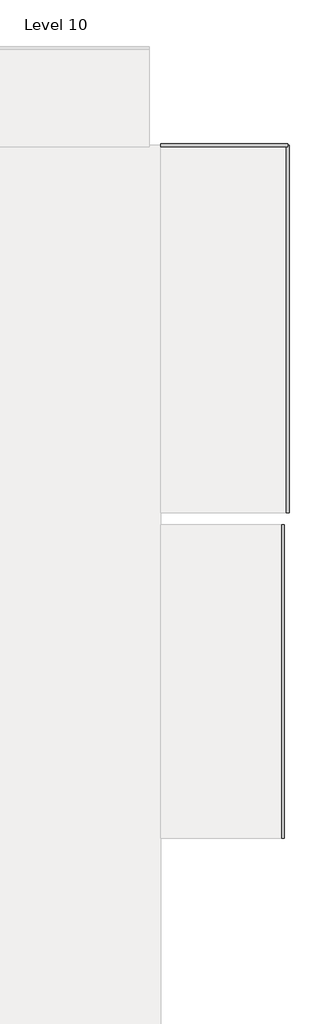
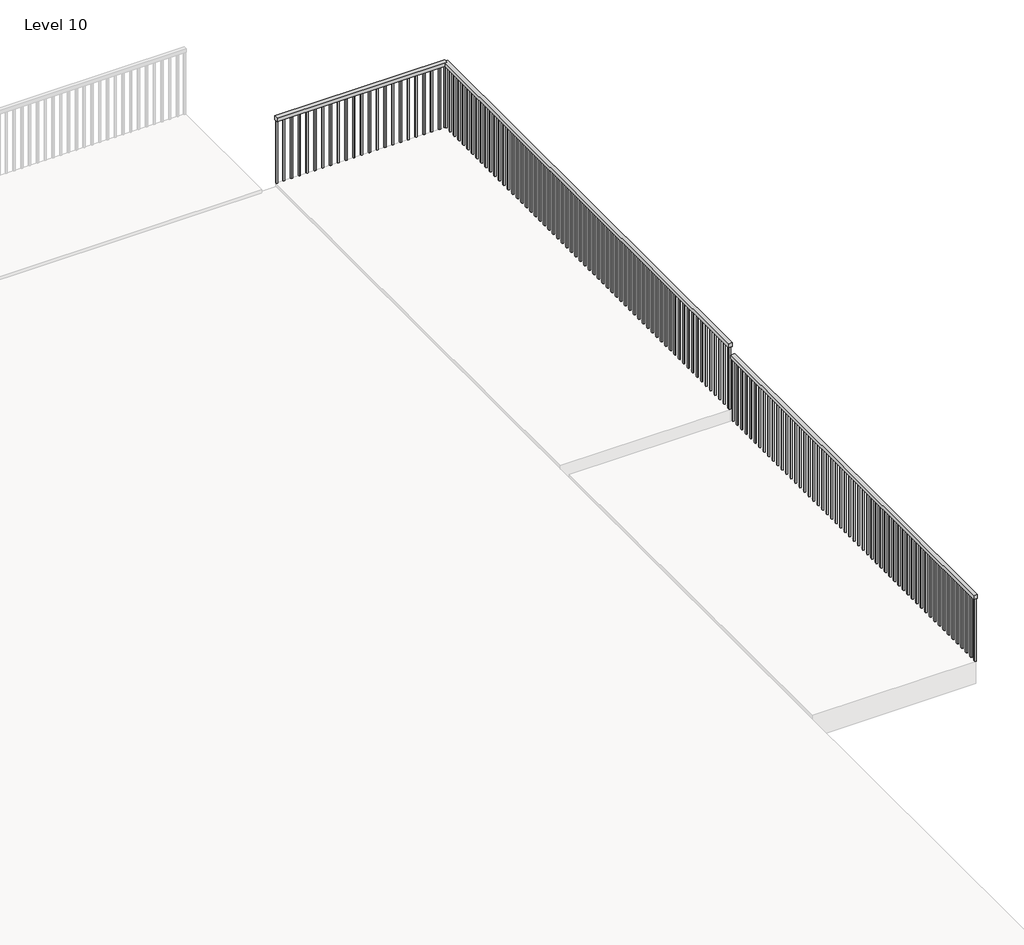
# One storey, part 4 of 5: 3 railings.
"""IFC4 building model written with IfcOpenShell, lengths in millimetres."""

from ifc_helpers import new_model, si_unit, frame, origin, place, context, project, spatial, polyline, outline, extrude, element, save

model = new_model("IFC4")

# Units and contexts
model_context = context("Model", 3, world=origin())
ifc_project = project(units=[si_unit("LENGTHUNIT", "METRE", prefix="MILLI")], contexts=[model_context])

# Site, building, storey
site = spatial("IfcSite", under=ifc_project)
building = spatial("IfcBuilding", under=site)
storey = spatial("IfcBuildingStorey", under=building, Name="Level 10", Elevation=12496.8)

# Railings
placement = place(None, origin())
element("IfcRailing", 1, ObjectType="Handrail - Rectangular", at=placement, inside=storey, context=model_context, shape_type="SweptSolid", body=[
    extrude(outline(polyline([(14106.5361222, 14772.744107), (14106.5361222, 14823.544107), (16321.4289933, 14823.544107), (16321.4289933, 14772.744107), (14106.5361222, 14772.744107)])), frame((0.0, 0.0, 13360.4), z_axis=(0.0, 0.0, 1.0), x_axis=(1.0, 0.0, 0.0)), (0.0, 0.0, 1.0), 50.8),
    extrude(outline(polyline([(16230.6111222, 14788.619107), (16230.6111222, 14807.669107), (16249.6611222, 14807.669107), (16249.6611222, 14788.619107), (16230.6111222, 14788.619107)])), frame((0.0, 0.0, 12496.8), z_axis=(0.0, 0.0, 1.0), x_axis=(1.0, 0.0, 0.0)), (0.0, 0.0, 1.0), 863.6),
    extrude(outline(polyline([(16129.0111222, 14788.619107), (16129.0111222, 14807.669107), (16148.0611222, 14807.669107), (16148.0611222, 14788.619107), (16129.0111222, 14788.619107)])), frame((0.0, 0.0, 12496.8), z_axis=(0.0, 0.0, 1.0), x_axis=(1.0, 0.0, 0.0)), (0.0, 0.0, 1.0), 863.6),
    extrude(outline(polyline([(16027.4111222, 14788.619107), (16027.4111222, 14807.669107), (16046.4611222, 14807.669107), (16046.4611222, 14788.619107), (16027.4111222, 14788.619107)])), frame((0.0, 0.0, 12496.8), z_axis=(0.0, 0.0, 1.0), x_axis=(1.0, 0.0, 0.0)), (0.0, 0.0, 1.0), 863.6),
    extrude(outline(polyline([(15925.8111222, 14788.619107), (15925.8111222, 14807.669107), (15944.8611222, 14807.669107), (15944.8611222, 14788.619107), (15925.8111222, 14788.619107)])), frame((0.0, 0.0, 12496.8), z_axis=(0.0, 0.0, 1.0), x_axis=(1.0, 0.0, 0.0)), (0.0, 0.0, 1.0), 863.6),
    extrude(outline(polyline([(15824.2111222, 14788.619107), (15824.2111222, 14807.669107), (15843.2611222, 14807.669107), (15843.2611222, 14788.619107), (15824.2111222, 14788.619107)])), frame((0.0, 0.0, 12496.8), z_axis=(0.0, 0.0, 1.0), x_axis=(1.0, 0.0, 0.0)), (0.0, 0.0, 1.0), 863.6),
    extrude(outline(polyline([(15722.6111222, 14788.619107), (15722.6111222, 14807.669107), (15741.6611222, 14807.669107), (15741.6611222, 14788.619107), (15722.6111222, 14788.619107)])), frame((0.0, 0.0, 12496.8), z_axis=(0.0, 0.0, 1.0), x_axis=(1.0, 0.0, 0.0)), (0.0, 0.0, 1.0), 863.6),
    extrude(outline(polyline([(15621.0111222, 14788.619107), (15621.0111222, 14807.669107), (15640.0611222, 14807.669107), (15640.0611222, 14788.619107), (15621.0111222, 14788.619107)])), frame((0.0, 0.0, 12496.8), z_axis=(0.0, 0.0, 1.0), x_axis=(1.0, 0.0, 0.0)), (0.0, 0.0, 1.0), 863.6),
    extrude(outline(polyline([(15519.4111222, 14788.619107), (15519.4111222, 14807.669107), (15538.4611222, 14807.669107), (15538.4611222, 14788.619107), (15519.4111222, 14788.619107)])), frame((0.0, 0.0, 12496.8), z_axis=(0.0, 0.0, 1.0), x_axis=(1.0, 0.0, 0.0)), (0.0, 0.0, 1.0), 863.6),
    extrude(outline(polyline([(15417.8111222, 14788.619107), (15417.8111222, 14807.669107), (15436.8611222, 14807.669107), (15436.8611222, 14788.619107), (15417.8111222, 14788.619107)])), frame((0.0, 0.0, 12496.8), z_axis=(0.0, 0.0, 1.0), x_axis=(1.0, 0.0, 0.0)), (0.0, 0.0, 1.0), 863.6),
    extrude(outline(polyline([(15316.2111222, 14788.619107), (15316.2111222, 14807.669107), (15335.2611222, 14807.669107), (15335.2611222, 14788.619107), (15316.2111222, 14788.619107)])), frame((0.0, 0.0, 12496.8), z_axis=(0.0, 0.0, 1.0), x_axis=(1.0, 0.0, 0.0)), (0.0, 0.0, 1.0), 863.6),
    extrude(outline(polyline([(15214.6111222, 14788.619107), (15214.6111222, 14807.669107), (15233.6611222, 14807.669107), (15233.6611222, 14788.619107), (15214.6111222, 14788.619107)])), frame((0.0, 0.0, 12496.8), z_axis=(0.0, 0.0, 1.0), x_axis=(1.0, 0.0, 0.0)), (0.0, 0.0, 1.0), 863.6),
    extrude(outline(polyline([(15113.0111222, 14788.619107), (15113.0111222, 14807.669107), (15132.0611222, 14807.669107), (15132.0611222, 14788.619107), (15113.0111222, 14788.619107)])), frame((0.0, 0.0, 12496.8), z_axis=(0.0, 0.0, 1.0), x_axis=(1.0, 0.0, 0.0)), (0.0, 0.0, 1.0), 863.6),
    extrude(outline(polyline([(15011.4111222, 14788.619107), (15011.4111222, 14807.669107), (15030.4611222, 14807.669107), (15030.4611222, 14788.619107), (15011.4111222, 14788.619107)])), frame((0.0, 0.0, 12496.8), z_axis=(0.0, 0.0, 1.0), x_axis=(1.0, 0.0, 0.0)), (0.0, 0.0, 1.0), 863.6),
    extrude(outline(polyline([(14909.8111222, 14788.619107), (14909.8111222, 14807.669107), (14928.8611222, 14807.669107), (14928.8611222, 14788.619107), (14909.8111222, 14788.619107)])), frame((0.0, 0.0, 12496.8), z_axis=(0.0, 0.0, 1.0), x_axis=(1.0, 0.0, 0.0)), (0.0, 0.0, 1.0), 863.6),
    extrude(outline(polyline([(14808.2111222, 14788.619107), (14808.2111222, 14807.669107), (14827.2611222, 14807.669107), (14827.2611222, 14788.619107), (14808.2111222, 14788.619107)])), frame((0.0, 0.0, 12496.8), z_axis=(0.0, 0.0, 1.0), x_axis=(1.0, 0.0, 0.0)), (0.0, 0.0, 1.0), 863.6),
    extrude(outline(polyline([(14706.6111222, 14788.619107), (14706.6111222, 14807.669107), (14725.6611222, 14807.669107), (14725.6611222, 14788.619107), (14706.6111222, 14788.619107)])), frame((0.0, 0.0, 12496.8), z_axis=(0.0, 0.0, 1.0), x_axis=(1.0, 0.0, 0.0)), (0.0, 0.0, 1.0), 863.6),
    extrude(outline(polyline([(14605.0111222, 14788.619107), (14605.0111222, 14807.669107), (14624.0611222, 14807.669107), (14624.0611222, 14788.619107), (14605.0111222, 14788.619107)])), frame((0.0, 0.0, 12496.8), z_axis=(0.0, 0.0, 1.0), x_axis=(1.0, 0.0, 0.0)), (0.0, 0.0, 1.0), 863.6),
    extrude(outline(polyline([(14503.4111222, 14788.619107), (14503.4111222, 14807.669107), (14522.4611222, 14807.669107), (14522.4611222, 14788.619107), (14503.4111222, 14788.619107)])), frame((0.0, 0.0, 12496.8), z_axis=(0.0, 0.0, 1.0), x_axis=(1.0, 0.0, 0.0)), (0.0, 0.0, 1.0), 863.6),
    extrude(outline(polyline([(14401.8111222, 14788.619107), (14401.8111222, 14807.669107), (14420.8611222, 14807.669107), (14420.8611222, 14788.619107), (14401.8111222, 14788.619107)])), frame((0.0, 0.0, 12496.8), z_axis=(0.0, 0.0, 1.0), x_axis=(1.0, 0.0, 0.0)), (0.0, 0.0, 1.0), 863.6),
    extrude(outline(polyline([(14300.2111222, 14788.619107), (14300.2111222, 14807.669107), (14319.2611222, 14807.669107), (14319.2611222, 14788.619107), (14300.2111222, 14788.619107)])), frame((0.0, 0.0, 12496.8), z_axis=(0.0, 0.0, 1.0), x_axis=(1.0, 0.0, 0.0)), (0.0, 0.0, 1.0), 863.6),
    extrude(outline(polyline([(14198.6111222, 14788.619107), (14198.6111222, 14807.669107), (14217.6611222, 14807.669107), (14217.6611222, 14788.619107), (14198.6111222, 14788.619107)])), frame((0.0, 0.0, 12496.8), z_axis=(0.0, 0.0, 1.0), x_axis=(1.0, 0.0, 0.0)), (0.0, 0.0, 1.0), 863.6),
    extrude(outline(polyline([(16302.3789933, 14788.619107), (16302.3789933, 14807.669107), (16321.4289933, 14807.669107), (16321.4289933, 14788.619107), (16302.3789933, 14788.619107)])), frame((0.0, 0.0, 12496.8), z_axis=(0.0, 0.0, 1.0), x_axis=(1.0, 0.0, 0.0)), (0.0, 0.0, 1.0), 863.6),
    extrude(outline(polyline([(14106.5361222, 14788.619107), (14106.5361222, 14807.669107), (14125.5861222, 14807.669107), (14125.5861222, 14788.619107), (14106.5361222, 14788.619107)])), frame((0.0, 0.0, 12496.8), z_axis=(0.0, 0.0, 1.0), x_axis=(1.0, 0.0, 0.0)), (0.0, 0.0, 1.0), 863.6),
])
element("IfcRailing", 2, ObjectType="Handrail - Rectangular", at=placement, inside=storey, context=model_context, shape_type="SweptSolid", body=[
    extrude(outline(polyline([(16296.0289933, 14798.144107), (16346.8289933, 14798.144107), (16346.8289933, 8367.8237525), (16296.0289933, 8367.8237525), (16296.0289933, 14798.144107)])), frame((0.0, 0.0, 13360.4), z_axis=(0.0, 0.0, 1.0), x_axis=(1.0, 0.0, 0.0)), (0.0, 0.0, 1.0), 50.8),
    extrude(outline(polyline([(16311.9039933, 8406.869107), (16330.9539933, 8406.869107), (16330.9539933, 8387.819107), (16311.9039933, 8387.819107), (16311.9039933, 8406.869107)])), frame((0.0, 0.0, 12496.8), z_axis=(0.0, 0.0, 1.0), x_axis=(1.0, 0.0, 0.0)), (0.0, 0.0, 1.0), 863.6),
    extrude(outline(polyline([(16311.9039933, 8508.469107), (16330.9539933, 8508.469107), (16330.9539933, 8489.419107), (16311.9039933, 8489.419107), (16311.9039933, 8508.469107)])), frame((0.0, 0.0, 12496.8), z_axis=(0.0, 0.0, 1.0), x_axis=(1.0, 0.0, 0.0)), (0.0, 0.0, 1.0), 863.6),
    extrude(outline(polyline([(16311.9039933, 8610.069107), (16330.9539933, 8610.069107), (16330.9539933, 8591.019107), (16311.9039933, 8591.019107), (16311.9039933, 8610.069107)])), frame((0.0, 0.0, 12496.8), z_axis=(0.0, 0.0, 1.0), x_axis=(1.0, 0.0, 0.0)), (0.0, 0.0, 1.0), 863.6),
    extrude(outline(polyline([(16311.9039933, 8711.669107), (16330.9539933, 8711.669107), (16330.9539933, 8692.619107), (16311.9039933, 8692.619107), (16311.9039933, 8711.669107)])), frame((0.0, 0.0, 12496.8), z_axis=(0.0, 0.0, 1.0), x_axis=(1.0, 0.0, 0.0)), (0.0, 0.0, 1.0), 863.6),
    extrude(outline(polyline([(16311.9039933, 8813.269107), (16330.9539933, 8813.269107), (16330.9539933, 8794.219107), (16311.9039933, 8794.219107), (16311.9039933, 8813.269107)])), frame((0.0, 0.0, 12496.8), z_axis=(0.0, 0.0, 1.0), x_axis=(1.0, 0.0, 0.0)), (0.0, 0.0, 1.0), 863.6),
    extrude(outline(polyline([(16311.9039933, 8914.869107), (16330.9539933, 8914.869107), (16330.9539933, 8895.819107), (16311.9039933, 8895.819107), (16311.9039933, 8914.869107)])), frame((0.0, 0.0, 12496.8), z_axis=(0.0, 0.0, 1.0), x_axis=(1.0, 0.0, 0.0)), (0.0, 0.0, 1.0), 863.6),
    extrude(outline(polyline([(16311.9039933, 9016.469107), (16330.9539933, 9016.469107), (16330.9539933, 8997.419107), (16311.9039933, 8997.419107), (16311.9039933, 9016.469107)])), frame((0.0, 0.0, 12496.8), z_axis=(0.0, 0.0, 1.0), x_axis=(1.0, 0.0, 0.0)), (0.0, 0.0, 1.0), 863.6),
    extrude(outline(polyline([(16311.9039933, 9118.069107), (16330.9539933, 9118.069107), (16330.9539933, 9099.019107), (16311.9039933, 9099.019107), (16311.9039933, 9118.069107)])), frame((0.0, 0.0, 12496.8), z_axis=(0.0, 0.0, 1.0), x_axis=(1.0, 0.0, 0.0)), (0.0, 0.0, 1.0), 863.6),
    extrude(outline(polyline([(16311.9039933, 9219.669107), (16330.9539933, 9219.669107), (16330.9539933, 9200.619107), (16311.9039933, 9200.619107), (16311.9039933, 9219.669107)])), frame((0.0, 0.0, 12496.8), z_axis=(0.0, 0.0, 1.0), x_axis=(1.0, 0.0, 0.0)), (0.0, 0.0, 1.0), 863.6),
    extrude(outline(polyline([(16311.9039933, 9321.269107), (16330.9539933, 9321.269107), (16330.9539933, 9302.219107), (16311.9039933, 9302.219107), (16311.9039933, 9321.269107)])), frame((0.0, 0.0, 12496.8), z_axis=(0.0, 0.0, 1.0), x_axis=(1.0, 0.0, 0.0)), (0.0, 0.0, 1.0), 863.6),
    extrude(outline(polyline([(16311.9039933, 9422.869107), (16330.9539933, 9422.869107), (16330.9539933, 9403.819107), (16311.9039933, 9403.819107), (16311.9039933, 9422.869107)])), frame((0.0, 0.0, 12496.8), z_axis=(0.0, 0.0, 1.0), x_axis=(1.0, 0.0, 0.0)), (0.0, 0.0, 1.0), 863.6),
    extrude(outline(polyline([(16311.9039933, 9524.469107), (16330.9539933, 9524.469107), (16330.9539933, 9505.419107), (16311.9039933, 9505.419107), (16311.9039933, 9524.469107)])), frame((0.0, 0.0, 12496.8), z_axis=(0.0, 0.0, 1.0), x_axis=(1.0, 0.0, 0.0)), (0.0, 0.0, 1.0), 863.6),
    extrude(outline(polyline([(16311.9039933, 9626.069107), (16330.9539933, 9626.069107), (16330.9539933, 9607.019107), (16311.9039933, 9607.019107), (16311.9039933, 9626.069107)])), frame((0.0, 0.0, 12496.8), z_axis=(0.0, 0.0, 1.0), x_axis=(1.0, 0.0, 0.0)), (0.0, 0.0, 1.0), 863.6),
    extrude(outline(polyline([(16311.9039933, 9727.669107), (16330.9539933, 9727.669107), (16330.9539933, 9708.619107), (16311.9039933, 9708.619107), (16311.9039933, 9727.669107)])), frame((0.0, 0.0, 12496.8), z_axis=(0.0, 0.0, 1.0), x_axis=(1.0, 0.0, 0.0)), (0.0, 0.0, 1.0), 863.6),
    extrude(outline(polyline([(16311.9039933, 9829.269107), (16330.9539933, 9829.269107), (16330.9539933, 9810.219107), (16311.9039933, 9810.219107), (16311.9039933, 9829.269107)])), frame((0.0, 0.0, 12496.8), z_axis=(0.0, 0.0, 1.0), x_axis=(1.0, 0.0, 0.0)), (0.0, 0.0, 1.0), 863.6),
    extrude(outline(polyline([(16311.9039933, 9930.869107), (16330.9539933, 9930.869107), (16330.9539933, 9911.819107), (16311.9039933, 9911.819107), (16311.9039933, 9930.869107)])), frame((0.0, 0.0, 12496.8), z_axis=(0.0, 0.0, 1.0), x_axis=(1.0, 0.0, 0.0)), (0.0, 0.0, 1.0), 863.6),
    extrude(outline(polyline([(16311.9039933, 10032.469107), (16330.9539933, 10032.469107), (16330.9539933, 10013.419107), (16311.9039933, 10013.419107), (16311.9039933, 10032.469107)])), frame((0.0, 0.0, 12496.8), z_axis=(0.0, 0.0, 1.0), x_axis=(1.0, 0.0, 0.0)), (0.0, 0.0, 1.0), 863.6),
    extrude(outline(polyline([(16311.9039933, 10134.069107), (16330.9539933, 10134.069107), (16330.9539933, 10115.019107), (16311.9039933, 10115.019107), (16311.9039933, 10134.069107)])), frame((0.0, 0.0, 12496.8), z_axis=(0.0, 0.0, 1.0), x_axis=(1.0, 0.0, 0.0)), (0.0, 0.0, 1.0), 863.6),
    extrude(outline(polyline([(16311.9039933, 10235.669107), (16330.9539933, 10235.669107), (16330.9539933, 10216.619107), (16311.9039933, 10216.619107), (16311.9039933, 10235.669107)])), frame((0.0, 0.0, 12496.8), z_axis=(0.0, 0.0, 1.0), x_axis=(1.0, 0.0, 0.0)), (0.0, 0.0, 1.0), 863.6),
    extrude(outline(polyline([(16311.9039933, 10337.269107), (16330.9539933, 10337.269107), (16330.9539933, 10318.219107), (16311.9039933, 10318.219107), (16311.9039933, 10337.269107)])), frame((0.0, 0.0, 12496.8), z_axis=(0.0, 0.0, 1.0), x_axis=(1.0, 0.0, 0.0)), (0.0, 0.0, 1.0), 863.6),
    extrude(outline(polyline([(16311.9039933, 10438.869107), (16330.9539933, 10438.869107), (16330.9539933, 10419.819107), (16311.9039933, 10419.819107), (16311.9039933, 10438.869107)])), frame((0.0, 0.0, 12496.8), z_axis=(0.0, 0.0, 1.0), x_axis=(1.0, 0.0, 0.0)), (0.0, 0.0, 1.0), 863.6),
    extrude(outline(polyline([(16311.9039933, 10540.469107), (16330.9539933, 10540.469107), (16330.9539933, 10521.419107), (16311.9039933, 10521.419107), (16311.9039933, 10540.469107)])), frame((0.0, 0.0, 12496.8), z_axis=(0.0, 0.0, 1.0), x_axis=(1.0, 0.0, 0.0)), (0.0, 0.0, 1.0), 863.6),
    extrude(outline(polyline([(16311.9039933, 10642.069107), (16330.9539933, 10642.069107), (16330.9539933, 10623.019107), (16311.9039933, 10623.019107), (16311.9039933, 10642.069107)])), frame((0.0, 0.0, 12496.8), z_axis=(0.0, 0.0, 1.0), x_axis=(1.0, 0.0, 0.0)), (0.0, 0.0, 1.0), 863.6),
    extrude(outline(polyline([(16311.9039933, 10743.669107), (16330.9539933, 10743.669107), (16330.9539933, 10724.619107), (16311.9039933, 10724.619107), (16311.9039933, 10743.669107)])), frame((0.0, 0.0, 12496.8), z_axis=(0.0, 0.0, 1.0), x_axis=(1.0, 0.0, 0.0)), (0.0, 0.0, 1.0), 863.6),
    extrude(outline(polyline([(16311.9039933, 10845.269107), (16330.9539933, 10845.269107), (16330.9539933, 10826.219107), (16311.9039933, 10826.219107), (16311.9039933, 10845.269107)])), frame((0.0, 0.0, 12496.8), z_axis=(0.0, 0.0, 1.0), x_axis=(1.0, 0.0, 0.0)), (0.0, 0.0, 1.0), 863.6),
    extrude(outline(polyline([(16311.9039933, 10946.869107), (16330.9539933, 10946.869107), (16330.9539933, 10927.819107), (16311.9039933, 10927.819107), (16311.9039933, 10946.869107)])), frame((0.0, 0.0, 12496.8), z_axis=(0.0, 0.0, 1.0), x_axis=(1.0, 0.0, 0.0)), (0.0, 0.0, 1.0), 863.6),
    extrude(outline(polyline([(16311.9039933, 11048.469107), (16330.9539933, 11048.469107), (16330.9539933, 11029.419107), (16311.9039933, 11029.419107), (16311.9039933, 11048.469107)])), frame((0.0, 0.0, 12496.8), z_axis=(0.0, 0.0, 1.0), x_axis=(1.0, 0.0, 0.0)), (0.0, 0.0, 1.0), 863.6),
    extrude(outline(polyline([(16311.9039933, 11150.069107), (16330.9539933, 11150.069107), (16330.9539933, 11131.019107), (16311.9039933, 11131.019107), (16311.9039933, 11150.069107)])), frame((0.0, 0.0, 12496.8), z_axis=(0.0, 0.0, 1.0), x_axis=(1.0, 0.0, 0.0)), (0.0, 0.0, 1.0), 863.6),
    extrude(outline(polyline([(16311.9039933, 11251.669107), (16330.9539933, 11251.669107), (16330.9539933, 11232.619107), (16311.9039933, 11232.619107), (16311.9039933, 11251.669107)])), frame((0.0, 0.0, 12496.8), z_axis=(0.0, 0.0, 1.0), x_axis=(1.0, 0.0, 0.0)), (0.0, 0.0, 1.0), 863.6),
    extrude(outline(polyline([(16311.9039933, 11353.269107), (16330.9539933, 11353.269107), (16330.9539933, 11334.219107), (16311.9039933, 11334.219107), (16311.9039933, 11353.269107)])), frame((0.0, 0.0, 12496.8), z_axis=(0.0, 0.0, 1.0), x_axis=(1.0, 0.0, 0.0)), (0.0, 0.0, 1.0), 863.6),
    extrude(outline(polyline([(16311.9039933, 11454.869107), (16330.9539933, 11454.869107), (16330.9539933, 11435.819107), (16311.9039933, 11435.819107), (16311.9039933, 11454.869107)])), frame((0.0, 0.0, 12496.8), z_axis=(0.0, 0.0, 1.0), x_axis=(1.0, 0.0, 0.0)), (0.0, 0.0, 1.0), 863.6),
    extrude(outline(polyline([(16311.9039933, 11556.469107), (16330.9539933, 11556.469107), (16330.9539933, 11537.419107), (16311.9039933, 11537.419107), (16311.9039933, 11556.469107)])), frame((0.0, 0.0, 12496.8), z_axis=(0.0, 0.0, 1.0), x_axis=(1.0, 0.0, 0.0)), (0.0, 0.0, 1.0), 863.6),
    extrude(outline(polyline([(16311.9039933, 11658.069107), (16330.9539933, 11658.069107), (16330.9539933, 11639.019107), (16311.9039933, 11639.019107), (16311.9039933, 11658.069107)])), frame((0.0, 0.0, 12496.8), z_axis=(0.0, 0.0, 1.0), x_axis=(1.0, 0.0, 0.0)), (0.0, 0.0, 1.0), 863.6),
    extrude(outline(polyline([(16311.9039933, 11759.669107), (16330.9539933, 11759.669107), (16330.9539933, 11740.619107), (16311.9039933, 11740.619107), (16311.9039933, 11759.669107)])), frame((0.0, 0.0, 12496.8), z_axis=(0.0, 0.0, 1.0), x_axis=(1.0, 0.0, 0.0)), (0.0, 0.0, 1.0), 863.6),
    extrude(outline(polyline([(16311.9039933, 11861.269107), (16330.9539933, 11861.269107), (16330.9539933, 11842.219107), (16311.9039933, 11842.219107), (16311.9039933, 11861.269107)])), frame((0.0, 0.0, 12496.8), z_axis=(0.0, 0.0, 1.0), x_axis=(1.0, 0.0, 0.0)), (0.0, 0.0, 1.0), 863.6),
    extrude(outline(polyline([(16311.9039933, 11962.869107), (16330.9539933, 11962.869107), (16330.9539933, 11943.819107), (16311.9039933, 11943.819107), (16311.9039933, 11962.869107)])), frame((0.0, 0.0, 12496.8), z_axis=(0.0, 0.0, 1.0), x_axis=(1.0, 0.0, 0.0)), (0.0, 0.0, 1.0), 863.6),
    extrude(outline(polyline([(16311.9039933, 12064.469107), (16330.9539933, 12064.469107), (16330.9539933, 12045.419107), (16311.9039933, 12045.419107), (16311.9039933, 12064.469107)])), frame((0.0, 0.0, 12496.8), z_axis=(0.0, 0.0, 1.0), x_axis=(1.0, 0.0, 0.0)), (0.0, 0.0, 1.0), 863.6),
    extrude(outline(polyline([(16311.9039933, 12166.069107), (16330.9539933, 12166.069107), (16330.9539933, 12147.019107), (16311.9039933, 12147.019107), (16311.9039933, 12166.069107)])), frame((0.0, 0.0, 12496.8), z_axis=(0.0, 0.0, 1.0), x_axis=(1.0, 0.0, 0.0)), (0.0, 0.0, 1.0), 863.6),
    extrude(outline(polyline([(16311.9039933, 12267.669107), (16330.9539933, 12267.669107), (16330.9539933, 12248.619107), (16311.9039933, 12248.619107), (16311.9039933, 12267.669107)])), frame((0.0, 0.0, 12496.8), z_axis=(0.0, 0.0, 1.0), x_axis=(1.0, 0.0, 0.0)), (0.0, 0.0, 1.0), 863.6),
    extrude(outline(polyline([(16311.9039933, 12369.269107), (16330.9539933, 12369.269107), (16330.9539933, 12350.219107), (16311.9039933, 12350.219107), (16311.9039933, 12369.269107)])), frame((0.0, 0.0, 12496.8), z_axis=(0.0, 0.0, 1.0), x_axis=(1.0, 0.0, 0.0)), (0.0, 0.0, 1.0), 863.6),
    extrude(outline(polyline([(16311.9039933, 12470.869107), (16330.9539933, 12470.869107), (16330.9539933, 12451.819107), (16311.9039933, 12451.819107), (16311.9039933, 12470.869107)])), frame((0.0, 0.0, 12496.8), z_axis=(0.0, 0.0, 1.0), x_axis=(1.0, 0.0, 0.0)), (0.0, 0.0, 1.0), 863.6),
    extrude(outline(polyline([(16311.9039933, 12572.469107), (16330.9539933, 12572.469107), (16330.9539933, 12553.419107), (16311.9039933, 12553.419107), (16311.9039933, 12572.469107)])), frame((0.0, 0.0, 12496.8), z_axis=(0.0, 0.0, 1.0), x_axis=(1.0, 0.0, 0.0)), (0.0, 0.0, 1.0), 863.6),
    extrude(outline(polyline([(16311.9039933, 12674.069107), (16330.9539933, 12674.069107), (16330.9539933, 12655.019107), (16311.9039933, 12655.019107), (16311.9039933, 12674.069107)])), frame((0.0, 0.0, 12496.8), z_axis=(0.0, 0.0, 1.0), x_axis=(1.0, 0.0, 0.0)), (0.0, 0.0, 1.0), 863.6),
    extrude(outline(polyline([(16311.9039933, 12775.669107), (16330.9539933, 12775.669107), (16330.9539933, 12756.619107), (16311.9039933, 12756.619107), (16311.9039933, 12775.669107)])), frame((0.0, 0.0, 12496.8), z_axis=(0.0, 0.0, 1.0), x_axis=(1.0, 0.0, 0.0)), (0.0, 0.0, 1.0), 863.6),
    extrude(outline(polyline([(16311.9039933, 12877.269107), (16330.9539933, 12877.269107), (16330.9539933, 12858.219107), (16311.9039933, 12858.219107), (16311.9039933, 12877.269107)])), frame((0.0, 0.0, 12496.8), z_axis=(0.0, 0.0, 1.0), x_axis=(1.0, 0.0, 0.0)), (0.0, 0.0, 1.0), 863.6),
    extrude(outline(polyline([(16311.9039933, 12978.869107), (16330.9539933, 12978.869107), (16330.9539933, 12959.819107), (16311.9039933, 12959.819107), (16311.9039933, 12978.869107)])), frame((0.0, 0.0, 12496.8), z_axis=(0.0, 0.0, 1.0), x_axis=(1.0, 0.0, 0.0)), (0.0, 0.0, 1.0), 863.6),
    extrude(outline(polyline([(16311.9039933, 13080.469107), (16330.9539933, 13080.469107), (16330.9539933, 13061.419107), (16311.9039933, 13061.419107), (16311.9039933, 13080.469107)])), frame((0.0, 0.0, 12496.8), z_axis=(0.0, 0.0, 1.0), x_axis=(1.0, 0.0, 0.0)), (0.0, 0.0, 1.0), 863.6),
    extrude(outline(polyline([(16311.9039933, 13182.069107), (16330.9539933, 13182.069107), (16330.9539933, 13163.019107), (16311.9039933, 13163.019107), (16311.9039933, 13182.069107)])), frame((0.0, 0.0, 12496.8), z_axis=(0.0, 0.0, 1.0), x_axis=(1.0, 0.0, 0.0)), (0.0, 0.0, 1.0), 863.6),
    extrude(outline(polyline([(16311.9039933, 13283.669107), (16330.9539933, 13283.669107), (16330.9539933, 13264.619107), (16311.9039933, 13264.619107), (16311.9039933, 13283.669107)])), frame((0.0, 0.0, 12496.8), z_axis=(0.0, 0.0, 1.0), x_axis=(1.0, 0.0, 0.0)), (0.0, 0.0, 1.0), 863.6),
    extrude(outline(polyline([(16311.9039933, 13385.269107), (16330.9539933, 13385.269107), (16330.9539933, 13366.219107), (16311.9039933, 13366.219107), (16311.9039933, 13385.269107)])), frame((0.0, 0.0, 12496.8), z_axis=(0.0, 0.0, 1.0), x_axis=(1.0, 0.0, 0.0)), (0.0, 0.0, 1.0), 863.6),
    extrude(outline(polyline([(16311.9039933, 13486.869107), (16330.9539933, 13486.869107), (16330.9539933, 13467.819107), (16311.9039933, 13467.819107), (16311.9039933, 13486.869107)])), frame((0.0, 0.0, 12496.8), z_axis=(0.0, 0.0, 1.0), x_axis=(1.0, 0.0, 0.0)), (0.0, 0.0, 1.0), 863.6),
    extrude(outline(polyline([(16311.9039933, 13588.469107), (16330.9539933, 13588.469107), (16330.9539933, 13569.419107), (16311.9039933, 13569.419107), (16311.9039933, 13588.469107)])), frame((0.0, 0.0, 12496.8), z_axis=(0.0, 0.0, 1.0), x_axis=(1.0, 0.0, 0.0)), (0.0, 0.0, 1.0), 863.6),
    extrude(outline(polyline([(16311.9039933, 13690.069107), (16330.9539933, 13690.069107), (16330.9539933, 13671.019107), (16311.9039933, 13671.019107), (16311.9039933, 13690.069107)])), frame((0.0, 0.0, 12496.8), z_axis=(0.0, 0.0, 1.0), x_axis=(1.0, 0.0, 0.0)), (0.0, 0.0, 1.0), 863.6),
    extrude(outline(polyline([(16311.9039933, 13791.669107), (16330.9539933, 13791.669107), (16330.9539933, 13772.619107), (16311.9039933, 13772.619107), (16311.9039933, 13791.669107)])), frame((0.0, 0.0, 12496.8), z_axis=(0.0, 0.0, 1.0), x_axis=(1.0, 0.0, 0.0)), (0.0, 0.0, 1.0), 863.6),
    extrude(outline(polyline([(16311.9039933, 13893.269107), (16330.9539933, 13893.269107), (16330.9539933, 13874.219107), (16311.9039933, 13874.219107), (16311.9039933, 13893.269107)])), frame((0.0, 0.0, 12496.8), z_axis=(0.0, 0.0, 1.0), x_axis=(1.0, 0.0, 0.0)), (0.0, 0.0, 1.0), 863.6),
    extrude(outline(polyline([(16311.9039933, 13994.869107), (16330.9539933, 13994.869107), (16330.9539933, 13975.819107), (16311.9039933, 13975.819107), (16311.9039933, 13994.869107)])), frame((0.0, 0.0, 12496.8), z_axis=(0.0, 0.0, 1.0), x_axis=(1.0, 0.0, 0.0)), (0.0, 0.0, 1.0), 863.6),
    extrude(outline(polyline([(16311.9039933, 14096.469107), (16330.9539933, 14096.469107), (16330.9539933, 14077.419107), (16311.9039933, 14077.419107), (16311.9039933, 14096.469107)])), frame((0.0, 0.0, 12496.8), z_axis=(0.0, 0.0, 1.0), x_axis=(1.0, 0.0, 0.0)), (0.0, 0.0, 1.0), 863.6),
    extrude(outline(polyline([(16311.9039933, 14198.069107), (16330.9539933, 14198.069107), (16330.9539933, 14179.019107), (16311.9039933, 14179.019107), (16311.9039933, 14198.069107)])), frame((0.0, 0.0, 12496.8), z_axis=(0.0, 0.0, 1.0), x_axis=(1.0, 0.0, 0.0)), (0.0, 0.0, 1.0), 863.6),
    extrude(outline(polyline([(16311.9039933, 14299.669107), (16330.9539933, 14299.669107), (16330.9539933, 14280.619107), (16311.9039933, 14280.619107), (16311.9039933, 14299.669107)])), frame((0.0, 0.0, 12496.8), z_axis=(0.0, 0.0, 1.0), x_axis=(1.0, 0.0, 0.0)), (0.0, 0.0, 1.0), 863.6),
    extrude(outline(polyline([(16311.9039933, 14401.269107), (16330.9539933, 14401.269107), (16330.9539933, 14382.219107), (16311.9039933, 14382.219107), (16311.9039933, 14401.269107)])), frame((0.0, 0.0, 12496.8), z_axis=(0.0, 0.0, 1.0), x_axis=(1.0, 0.0, 0.0)), (0.0, 0.0, 1.0), 863.6),
    extrude(outline(polyline([(16311.9039933, 14502.869107), (16330.9539933, 14502.869107), (16330.9539933, 14483.819107), (16311.9039933, 14483.819107), (16311.9039933, 14502.869107)])), frame((0.0, 0.0, 12496.8), z_axis=(0.0, 0.0, 1.0), x_axis=(1.0, 0.0, 0.0)), (0.0, 0.0, 1.0), 863.6),
    extrude(outline(polyline([(16311.9039933, 14604.469107), (16330.9539933, 14604.469107), (16330.9539933, 14585.419107), (16311.9039933, 14585.419107), (16311.9039933, 14604.469107)])), frame((0.0, 0.0, 12496.8), z_axis=(0.0, 0.0, 1.0), x_axis=(1.0, 0.0, 0.0)), (0.0, 0.0, 1.0), 863.6),
    extrude(outline(polyline([(16311.9039933, 14706.069107), (16330.9539933, 14706.069107), (16330.9539933, 14687.019107), (16311.9039933, 14687.019107), (16311.9039933, 14706.069107)])), frame((0.0, 0.0, 12496.8), z_axis=(0.0, 0.0, 1.0), x_axis=(1.0, 0.0, 0.0)), (0.0, 0.0, 1.0), 863.6),
    extrude(outline(polyline([(16311.9039933, 8386.8737525), (16330.9539933, 8386.8737525), (16330.9539933, 8367.8237525), (16311.9039933, 8367.8237525), (16311.9039933, 8386.8737525)])), frame((0.0, 0.0, 12496.8), z_axis=(0.0, 0.0, 1.0), x_axis=(1.0, 0.0, 0.0)), (0.0, 0.0, 1.0), 863.6),
    extrude(outline(polyline([(16311.9039933, 14798.144107), (16330.9539933, 14798.144107), (16330.9539933, 14779.094107), (16311.9039933, 14779.094107), (16311.9039933, 14798.144107)])), frame((0.0, 0.0, 12496.8), z_axis=(0.0, 0.0, 1.0), x_axis=(1.0, 0.0, 0.0)), (0.0, 0.0, 1.0), 863.6),
])
element("IfcRailing", 3, ObjectType="Handrail - Rectangular", at=placement, inside=storey, context=model_context, shape_type="SweptSolid", body=[
    extrude(outline(polyline([(16214.7361222, 8164.6237525), (16265.5361222, 8164.6237525), (16265.5361222, 2678.2237525), (16214.7361222, 2678.2237525), (16214.7361222, 8164.6237525)])), frame((0.0, 0.0, 13360.4), z_axis=(0.0, 0.0, 1.0), x_axis=(1.0, 0.0, 0.0)), (0.0, 0.0, 1.0), 50.8),
    extrude(outline(polyline([(16230.6111222, 2789.3487525), (16249.6611222, 2789.3487525), (16249.6611222, 2770.2987525), (16230.6111222, 2770.2987525), (16230.6111222, 2789.3487525)])), frame((0.0, 0.0, 12496.8), z_axis=(0.0, 0.0, 1.0), x_axis=(1.0, 0.0, 0.0)), (0.0, 0.0, 1.0), 863.6),
    extrude(outline(polyline([(16230.6111222, 2890.9487525), (16249.6611222, 2890.9487525), (16249.6611222, 2871.8987525), (16230.6111222, 2871.8987525), (16230.6111222, 2890.9487525)])), frame((0.0, 0.0, 12496.8), z_axis=(0.0, 0.0, 1.0), x_axis=(1.0, 0.0, 0.0)), (0.0, 0.0, 1.0), 863.6),
    extrude(outline(polyline([(16230.6111222, 2992.5487525), (16249.6611222, 2992.5487525), (16249.6611222, 2973.4987525), (16230.6111222, 2973.4987525), (16230.6111222, 2992.5487525)])), frame((0.0, 0.0, 12496.8), z_axis=(0.0, 0.0, 1.0), x_axis=(1.0, 0.0, 0.0)), (0.0, 0.0, 1.0), 863.6),
    extrude(outline(polyline([(16230.6111222, 3094.1487525), (16249.6611222, 3094.1487525), (16249.6611222, 3075.0987525), (16230.6111222, 3075.0987525), (16230.6111222, 3094.1487525)])), frame((0.0, 0.0, 12496.8), z_axis=(0.0, 0.0, 1.0), x_axis=(1.0, 0.0, 0.0)), (0.0, 0.0, 1.0), 863.6),
    extrude(outline(polyline([(16230.6111222, 3195.7487525), (16249.6611222, 3195.7487525), (16249.6611222, 3176.6987525), (16230.6111222, 3176.6987525), (16230.6111222, 3195.7487525)])), frame((0.0, 0.0, 12496.8), z_axis=(0.0, 0.0, 1.0), x_axis=(1.0, 0.0, 0.0)), (0.0, 0.0, 1.0), 863.6),
    extrude(outline(polyline([(16230.6111222, 3297.3487525), (16249.6611222, 3297.3487525), (16249.6611222, 3278.2987525), (16230.6111222, 3278.2987525), (16230.6111222, 3297.3487525)])), frame((0.0, 0.0, 12496.8), z_axis=(0.0, 0.0, 1.0), x_axis=(1.0, 0.0, 0.0)), (0.0, 0.0, 1.0), 863.6),
    extrude(outline(polyline([(16230.6111222, 3398.9487525), (16249.6611222, 3398.9487525), (16249.6611222, 3379.8987525), (16230.6111222, 3379.8987525), (16230.6111222, 3398.9487525)])), frame((0.0, 0.0, 12496.8), z_axis=(0.0, 0.0, 1.0), x_axis=(1.0, 0.0, 0.0)), (0.0, 0.0, 1.0), 863.6),
    extrude(outline(polyline([(16230.6111222, 3500.5487525), (16249.6611222, 3500.5487525), (16249.6611222, 3481.4987525), (16230.6111222, 3481.4987525), (16230.6111222, 3500.5487525)])), frame((0.0, 0.0, 12496.8), z_axis=(0.0, 0.0, 1.0), x_axis=(1.0, 0.0, 0.0)), (0.0, 0.0, 1.0), 863.6),
    extrude(outline(polyline([(16230.6111222, 3602.1487525), (16249.6611222, 3602.1487525), (16249.6611222, 3583.0987525), (16230.6111222, 3583.0987525), (16230.6111222, 3602.1487525)])), frame((0.0, 0.0, 12496.8), z_axis=(0.0, 0.0, 1.0), x_axis=(1.0, 0.0, 0.0)), (0.0, 0.0, 1.0), 863.6),
    extrude(outline(polyline([(16230.6111222, 3703.7487525), (16249.6611222, 3703.7487525), (16249.6611222, 3684.6987525), (16230.6111222, 3684.6987525), (16230.6111222, 3703.7487525)])), frame((0.0, 0.0, 12496.8), z_axis=(0.0, 0.0, 1.0), x_axis=(1.0, 0.0, 0.0)), (0.0, 0.0, 1.0), 863.6),
    extrude(outline(polyline([(16230.6111222, 3805.3487525), (16249.6611222, 3805.3487525), (16249.6611222, 3786.2987525), (16230.6111222, 3786.2987525), (16230.6111222, 3805.3487525)])), frame((0.0, 0.0, 12496.8), z_axis=(0.0, 0.0, 1.0), x_axis=(1.0, 0.0, 0.0)), (0.0, 0.0, 1.0), 863.6),
    extrude(outline(polyline([(16230.6111222, 3906.9487525), (16249.6611222, 3906.9487525), (16249.6611222, 3887.8987525), (16230.6111222, 3887.8987525), (16230.6111222, 3906.9487525)])), frame((0.0, 0.0, 12496.8), z_axis=(0.0, 0.0, 1.0), x_axis=(1.0, 0.0, 0.0)), (0.0, 0.0, 1.0), 863.6),
    extrude(outline(polyline([(16230.6111222, 4008.5487525), (16249.6611222, 4008.5487525), (16249.6611222, 3989.4987525), (16230.6111222, 3989.4987525), (16230.6111222, 4008.5487525)])), frame((0.0, 0.0, 12496.8), z_axis=(0.0, 0.0, 1.0), x_axis=(1.0, 0.0, 0.0)), (0.0, 0.0, 1.0), 863.6),
    extrude(outline(polyline([(16230.6111222, 4110.1487525), (16249.6611222, 4110.1487525), (16249.6611222, 4091.0987525), (16230.6111222, 4091.0987525), (16230.6111222, 4110.1487525)])), frame((0.0, 0.0, 12496.8), z_axis=(0.0, 0.0, 1.0), x_axis=(1.0, 0.0, 0.0)), (0.0, 0.0, 1.0), 863.6),
    extrude(outline(polyline([(16230.6111222, 4211.7487525), (16249.6611222, 4211.7487525), (16249.6611222, 4192.6987525), (16230.6111222, 4192.6987525), (16230.6111222, 4211.7487525)])), frame((0.0, 0.0, 12496.8), z_axis=(0.0, 0.0, 1.0), x_axis=(1.0, 0.0, 0.0)), (0.0, 0.0, 1.0), 863.6),
    extrude(outline(polyline([(16230.6111222, 4313.3487525), (16249.6611222, 4313.3487525), (16249.6611222, 4294.2987525), (16230.6111222, 4294.2987525), (16230.6111222, 4313.3487525)])), frame((0.0, 0.0, 12496.8), z_axis=(0.0, 0.0, 1.0), x_axis=(1.0, 0.0, 0.0)), (0.0, 0.0, 1.0), 863.6),
    extrude(outline(polyline([(16230.6111222, 4414.9487525), (16249.6611222, 4414.9487525), (16249.6611222, 4395.8987525), (16230.6111222, 4395.8987525), (16230.6111222, 4414.9487525)])), frame((0.0, 0.0, 12496.8), z_axis=(0.0, 0.0, 1.0), x_axis=(1.0, 0.0, 0.0)), (0.0, 0.0, 1.0), 863.6),
    extrude(outline(polyline([(16230.6111222, 4516.5487525), (16249.6611222, 4516.5487525), (16249.6611222, 4497.4987525), (16230.6111222, 4497.4987525), (16230.6111222, 4516.5487525)])), frame((0.0, 0.0, 12496.8), z_axis=(0.0, 0.0, 1.0), x_axis=(1.0, 0.0, 0.0)), (0.0, 0.0, 1.0), 863.6),
    extrude(outline(polyline([(16230.6111222, 4618.1487525), (16249.6611222, 4618.1487525), (16249.6611222, 4599.0987525), (16230.6111222, 4599.0987525), (16230.6111222, 4618.1487525)])), frame((0.0, 0.0, 12496.8), z_axis=(0.0, 0.0, 1.0), x_axis=(1.0, 0.0, 0.0)), (0.0, 0.0, 1.0), 863.6),
    extrude(outline(polyline([(16230.6111222, 4719.7487525), (16249.6611222, 4719.7487525), (16249.6611222, 4700.6987525), (16230.6111222, 4700.6987525), (16230.6111222, 4719.7487525)])), frame((0.0, 0.0, 12496.8), z_axis=(0.0, 0.0, 1.0), x_axis=(1.0, 0.0, 0.0)), (0.0, 0.0, 1.0), 863.6),
    extrude(outline(polyline([(16230.6111222, 4821.3487525), (16249.6611222, 4821.3487525), (16249.6611222, 4802.2987525), (16230.6111222, 4802.2987525), (16230.6111222, 4821.3487525)])), frame((0.0, 0.0, 12496.8), z_axis=(0.0, 0.0, 1.0), x_axis=(1.0, 0.0, 0.0)), (0.0, 0.0, 1.0), 863.6),
    extrude(outline(polyline([(16230.6111222, 4922.9487525), (16249.6611222, 4922.9487525), (16249.6611222, 4903.8987525), (16230.6111222, 4903.8987525), (16230.6111222, 4922.9487525)])), frame((0.0, 0.0, 12496.8), z_axis=(0.0, 0.0, 1.0), x_axis=(1.0, 0.0, 0.0)), (0.0, 0.0, 1.0), 863.6),
    extrude(outline(polyline([(16230.6111222, 5024.5487525), (16249.6611222, 5024.5487525), (16249.6611222, 5005.4987525), (16230.6111222, 5005.4987525), (16230.6111222, 5024.5487525)])), frame((0.0, 0.0, 12496.8), z_axis=(0.0, 0.0, 1.0), x_axis=(1.0, 0.0, 0.0)), (0.0, 0.0, 1.0), 863.6),
    extrude(outline(polyline([(16230.6111222, 5126.1487525), (16249.6611222, 5126.1487525), (16249.6611222, 5107.0987525), (16230.6111222, 5107.0987525), (16230.6111222, 5126.1487525)])), frame((0.0, 0.0, 12496.8), z_axis=(0.0, 0.0, 1.0), x_axis=(1.0, 0.0, 0.0)), (0.0, 0.0, 1.0), 863.6),
    extrude(outline(polyline([(16230.6111222, 5227.7487525), (16249.6611222, 5227.7487525), (16249.6611222, 5208.6987525), (16230.6111222, 5208.6987525), (16230.6111222, 5227.7487525)])), frame((0.0, 0.0, 12496.8), z_axis=(0.0, 0.0, 1.0), x_axis=(1.0, 0.0, 0.0)), (0.0, 0.0, 1.0), 863.6),
    extrude(outline(polyline([(16230.6111222, 5329.3487525), (16249.6611222, 5329.3487525), (16249.6611222, 5310.2987525), (16230.6111222, 5310.2987525), (16230.6111222, 5329.3487525)])), frame((0.0, 0.0, 12496.8), z_axis=(0.0, 0.0, 1.0), x_axis=(1.0, 0.0, 0.0)), (0.0, 0.0, 1.0), 863.6),
    extrude(outline(polyline([(16230.6111222, 5430.9487525), (16249.6611222, 5430.9487525), (16249.6611222, 5411.8987525), (16230.6111222, 5411.8987525), (16230.6111222, 5430.9487525)])), frame((0.0, 0.0, 12496.8), z_axis=(0.0, 0.0, 1.0), x_axis=(1.0, 0.0, 0.0)), (0.0, 0.0, 1.0), 863.6),
    extrude(outline(polyline([(16230.6111222, 5532.5487525), (16249.6611222, 5532.5487525), (16249.6611222, 5513.4987525), (16230.6111222, 5513.4987525), (16230.6111222, 5532.5487525)])), frame((0.0, 0.0, 12496.8), z_axis=(0.0, 0.0, 1.0), x_axis=(1.0, 0.0, 0.0)), (0.0, 0.0, 1.0), 863.6),
    extrude(outline(polyline([(16230.6111222, 5634.1487525), (16249.6611222, 5634.1487525), (16249.6611222, 5615.0987525), (16230.6111222, 5615.0987525), (16230.6111222, 5634.1487525)])), frame((0.0, 0.0, 12496.8), z_axis=(0.0, 0.0, 1.0), x_axis=(1.0, 0.0, 0.0)), (0.0, 0.0, 1.0), 863.6),
    extrude(outline(polyline([(16230.6111222, 5735.7487525), (16249.6611222, 5735.7487525), (16249.6611222, 5716.6987525), (16230.6111222, 5716.6987525), (16230.6111222, 5735.7487525)])), frame((0.0, 0.0, 12496.8), z_axis=(0.0, 0.0, 1.0), x_axis=(1.0, 0.0, 0.0)), (0.0, 0.0, 1.0), 863.6),
    extrude(outline(polyline([(16230.6111222, 5837.3487525), (16249.6611222, 5837.3487525), (16249.6611222, 5818.2987525), (16230.6111222, 5818.2987525), (16230.6111222, 5837.3487525)])), frame((0.0, 0.0, 12496.8), z_axis=(0.0, 0.0, 1.0), x_axis=(1.0, 0.0, 0.0)), (0.0, 0.0, 1.0), 863.6),
    extrude(outline(polyline([(16230.6111222, 5938.9487525), (16249.6611222, 5938.9487525), (16249.6611222, 5919.8987525), (16230.6111222, 5919.8987525), (16230.6111222, 5938.9487525)])), frame((0.0, 0.0, 12496.8), z_axis=(0.0, 0.0, 1.0), x_axis=(1.0, 0.0, 0.0)), (0.0, 0.0, 1.0), 863.6),
    extrude(outline(polyline([(16230.6111222, 6040.5487525), (16249.6611222, 6040.5487525), (16249.6611222, 6021.4987525), (16230.6111222, 6021.4987525), (16230.6111222, 6040.5487525)])), frame((0.0, 0.0, 12496.8), z_axis=(0.0, 0.0, 1.0), x_axis=(1.0, 0.0, 0.0)), (0.0, 0.0, 1.0), 863.6),
    extrude(outline(polyline([(16230.6111222, 6142.1487525), (16249.6611222, 6142.1487525), (16249.6611222, 6123.0987525), (16230.6111222, 6123.0987525), (16230.6111222, 6142.1487525)])), frame((0.0, 0.0, 12496.8), z_axis=(0.0, 0.0, 1.0), x_axis=(1.0, 0.0, 0.0)), (0.0, 0.0, 1.0), 863.6),
    extrude(outline(polyline([(16230.6111222, 6243.7487525), (16249.6611222, 6243.7487525), (16249.6611222, 6224.6987525), (16230.6111222, 6224.6987525), (16230.6111222, 6243.7487525)])), frame((0.0, 0.0, 12496.8), z_axis=(0.0, 0.0, 1.0), x_axis=(1.0, 0.0, 0.0)), (0.0, 0.0, 1.0), 863.6),
    extrude(outline(polyline([(16230.6111222, 6345.3487525), (16249.6611222, 6345.3487525), (16249.6611222, 6326.2987525), (16230.6111222, 6326.2987525), (16230.6111222, 6345.3487525)])), frame((0.0, 0.0, 12496.8), z_axis=(0.0, 0.0, 1.0), x_axis=(1.0, 0.0, 0.0)), (0.0, 0.0, 1.0), 863.6),
    extrude(outline(polyline([(16230.6111222, 6446.9487525), (16249.6611222, 6446.9487525), (16249.6611222, 6427.8987525), (16230.6111222, 6427.8987525), (16230.6111222, 6446.9487525)])), frame((0.0, 0.0, 12496.8), z_axis=(0.0, 0.0, 1.0), x_axis=(1.0, 0.0, 0.0)), (0.0, 0.0, 1.0), 863.6),
    extrude(outline(polyline([(16230.6111222, 6548.5487525), (16249.6611222, 6548.5487525), (16249.6611222, 6529.4987525), (16230.6111222, 6529.4987525), (16230.6111222, 6548.5487525)])), frame((0.0, 0.0, 12496.8), z_axis=(0.0, 0.0, 1.0), x_axis=(1.0, 0.0, 0.0)), (0.0, 0.0, 1.0), 863.6),
    extrude(outline(polyline([(16230.6111222, 6650.1487525), (16249.6611222, 6650.1487525), (16249.6611222, 6631.0987525), (16230.6111222, 6631.0987525), (16230.6111222, 6650.1487525)])), frame((0.0, 0.0, 12496.8), z_axis=(0.0, 0.0, 1.0), x_axis=(1.0, 0.0, 0.0)), (0.0, 0.0, 1.0), 863.6),
    extrude(outline(polyline([(16230.6111222, 6751.7487525), (16249.6611222, 6751.7487525), (16249.6611222, 6732.6987525), (16230.6111222, 6732.6987525), (16230.6111222, 6751.7487525)])), frame((0.0, 0.0, 12496.8), z_axis=(0.0, 0.0, 1.0), x_axis=(1.0, 0.0, 0.0)), (0.0, 0.0, 1.0), 863.6),
    extrude(outline(polyline([(16230.6111222, 6853.3487525), (16249.6611222, 6853.3487525), (16249.6611222, 6834.2987525), (16230.6111222, 6834.2987525), (16230.6111222, 6853.3487525)])), frame((0.0, 0.0, 12496.8), z_axis=(0.0, 0.0, 1.0), x_axis=(1.0, 0.0, 0.0)), (0.0, 0.0, 1.0), 863.6),
    extrude(outline(polyline([(16230.6111222, 6954.9487525), (16249.6611222, 6954.9487525), (16249.6611222, 6935.8987525), (16230.6111222, 6935.8987525), (16230.6111222, 6954.9487525)])), frame((0.0, 0.0, 12496.8), z_axis=(0.0, 0.0, 1.0), x_axis=(1.0, 0.0, 0.0)), (0.0, 0.0, 1.0), 863.6),
    extrude(outline(polyline([(16230.6111222, 7056.5487525), (16249.6611222, 7056.5487525), (16249.6611222, 7037.4987525), (16230.6111222, 7037.4987525), (16230.6111222, 7056.5487525)])), frame((0.0, 0.0, 12496.8), z_axis=(0.0, 0.0, 1.0), x_axis=(1.0, 0.0, 0.0)), (0.0, 0.0, 1.0), 863.6),
    extrude(outline(polyline([(16230.6111222, 7158.1487525), (16249.6611222, 7158.1487525), (16249.6611222, 7139.0987525), (16230.6111222, 7139.0987525), (16230.6111222, 7158.1487525)])), frame((0.0, 0.0, 12496.8), z_axis=(0.0, 0.0, 1.0), x_axis=(1.0, 0.0, 0.0)), (0.0, 0.0, 1.0), 863.6),
    extrude(outline(polyline([(16230.6111222, 7259.7487525), (16249.6611222, 7259.7487525), (16249.6611222, 7240.6987525), (16230.6111222, 7240.6987525), (16230.6111222, 7259.7487525)])), frame((0.0, 0.0, 12496.8), z_axis=(0.0, 0.0, 1.0), x_axis=(1.0, 0.0, 0.0)), (0.0, 0.0, 1.0), 863.6),
    extrude(outline(polyline([(16230.6111222, 7361.3487525), (16249.6611222, 7361.3487525), (16249.6611222, 7342.2987525), (16230.6111222, 7342.2987525), (16230.6111222, 7361.3487525)])), frame((0.0, 0.0, 12496.8), z_axis=(0.0, 0.0, 1.0), x_axis=(1.0, 0.0, 0.0)), (0.0, 0.0, 1.0), 863.6),
    extrude(outline(polyline([(16230.6111222, 7462.9487525), (16249.6611222, 7462.9487525), (16249.6611222, 7443.8987525), (16230.6111222, 7443.8987525), (16230.6111222, 7462.9487525)])), frame((0.0, 0.0, 12496.8), z_axis=(0.0, 0.0, 1.0), x_axis=(1.0, 0.0, 0.0)), (0.0, 0.0, 1.0), 863.6),
    extrude(outline(polyline([(16230.6111222, 7564.5487525), (16249.6611222, 7564.5487525), (16249.6611222, 7545.4987525), (16230.6111222, 7545.4987525), (16230.6111222, 7564.5487525)])), frame((0.0, 0.0, 12496.8), z_axis=(0.0, 0.0, 1.0), x_axis=(1.0, 0.0, 0.0)), (0.0, 0.0, 1.0), 863.6),
    extrude(outline(polyline([(16230.6111222, 7666.1487525), (16249.6611222, 7666.1487525), (16249.6611222, 7647.0987525), (16230.6111222, 7647.0987525), (16230.6111222, 7666.1487525)])), frame((0.0, 0.0, 12496.8), z_axis=(0.0, 0.0, 1.0), x_axis=(1.0, 0.0, 0.0)), (0.0, 0.0, 1.0), 863.6),
    extrude(outline(polyline([(16230.6111222, 7767.7487525), (16249.6611222, 7767.7487525), (16249.6611222, 7748.6987525), (16230.6111222, 7748.6987525), (16230.6111222, 7767.7487525)])), frame((0.0, 0.0, 12496.8), z_axis=(0.0, 0.0, 1.0), x_axis=(1.0, 0.0, 0.0)), (0.0, 0.0, 1.0), 863.6),
    extrude(outline(polyline([(16230.6111222, 7869.3487525), (16249.6611222, 7869.3487525), (16249.6611222, 7850.2987525), (16230.6111222, 7850.2987525), (16230.6111222, 7869.3487525)])), frame((0.0, 0.0, 12496.8), z_axis=(0.0, 0.0, 1.0), x_axis=(1.0, 0.0, 0.0)), (0.0, 0.0, 1.0), 863.6),
    extrude(outline(polyline([(16230.6111222, 7970.9487525), (16249.6611222, 7970.9487525), (16249.6611222, 7951.8987525), (16230.6111222, 7951.8987525), (16230.6111222, 7970.9487525)])), frame((0.0, 0.0, 12496.8), z_axis=(0.0, 0.0, 1.0), x_axis=(1.0, 0.0, 0.0)), (0.0, 0.0, 1.0), 863.6),
    extrude(outline(polyline([(16230.6111222, 8072.5487525), (16249.6611222, 8072.5487525), (16249.6611222, 8053.4987525), (16230.6111222, 8053.4987525), (16230.6111222, 8072.5487525)])), frame((0.0, 0.0, 12496.8), z_axis=(0.0, 0.0, 1.0), x_axis=(1.0, 0.0, 0.0)), (0.0, 0.0, 1.0), 863.6),
    extrude(outline(polyline([(16230.6111222, 2697.2737525), (16249.6611222, 2697.2737525), (16249.6611222, 2678.2237525), (16230.6111222, 2678.2237525), (16230.6111222, 2697.2737525)])), frame((0.0, 0.0, 12496.8), z_axis=(0.0, 0.0, 1.0), x_axis=(1.0, 0.0, 0.0)), (0.0, 0.0, 1.0), 863.6),
    extrude(outline(polyline([(16230.6111222, 8164.6237525), (16249.6611222, 8164.6237525), (16249.6611222, 8145.5737525), (16230.6111222, 8145.5737525), (16230.6111222, 8164.6237525)])), frame((0.0, 0.0, 12496.8), z_axis=(0.0, 0.0, 1.0), x_axis=(1.0, 0.0, 0.0)), (0.0, 0.0, 1.0), 863.6),
])

save(model, "model.ifc")

# Revit data of these elements
# Type "Handrail - Rectangular"
#   Assembly Code = "C2010400"
#   built-in parameter 1008612 = 0.0416667 (stored number, unit not read)
#   built-in parameter 1008611 = 0.0416667 (stored number, unit not read)
#   built-in parameter 1008609 = 0.333333 (stored number, unit not read)
#   built-in parameter 1008604 = 0.166667 (stored number, unit not read)
#   built-in parameter 1008603 = 0.166667 (stored number, unit not read)
#   Railing Height = 3' - 0"
#   built-in parameter 1008630 = 2
#   built-in parameter 1008610 = 2
#   built-in parameter 1008618 = Baluster - Square : 3/4"
# Elements 1, 2, 3 (IfcRailing, "Handrail - Rectangular")
#   Phase Created = New Construction
